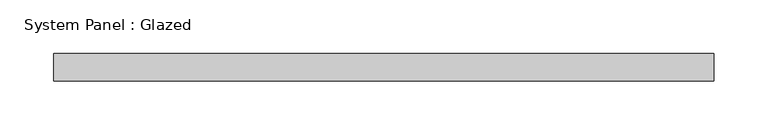
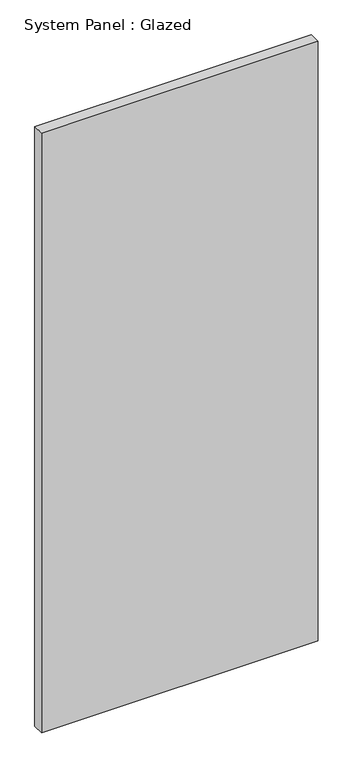
"""IFC4 building model written with IfcOpenShell, lengths in millimetres: plate geometry, System Panel : Glazed."""

from ifc_helpers import new_model, si_unit, origin, origin_with_axes, place, context, project, spatial, polyline, outline, extrude, source, transform, mapped, element, save


def system_panel_glazed_4048e9f5(model_context):
    return source(origin(), model_context, "Body", "SweptSolid", [
        extrude(outline(polyline([(306.3875, 19.05), (-306.3875, 19.05), (-306.3875, 44.45), (306.3875, 44.45), (306.3875, 19.05)])), origin_with_axes(), (0.0, 0.0, 1.0), 1404.3368617),
    ])


if __name__ == "__main__":
    model = new_model("IFC4")
    model_context = context("Model", 3, world=origin())
    ifc_project = project(units=[si_unit("LENGTHUNIT", "METRE", prefix="MILLI")], contexts=[model_context])
    site = spatial("IfcSite", under=ifc_project)
    building = spatial("IfcBuilding", under=site)
    placement = place(None, origin())
    system_panel_glazed_shape = system_panel_glazed_4048e9f5(model_context)
    element("IfcPlate", 1, ObjectType="System Panel : Glazed", at=placement, inside=building, context=model_context, shape_type="MappedRepresentation", body=[
        mapped(system_panel_glazed_shape, transform((0.0, 0.0, 0.0), x_axis=(1.0, 0.0, 0.0), y_axis=(0.0, 1.0, 0.0), z_axis=(0.0, 0.0, 1.0))),
    ])
    save(model, "model.ifc")

# Revit data of these elements
# Type "System Panel : Glazed"
#   Construction Type Id = "GSP4R"
#   Analytic Construction = "1/8 in Pilkington single glazing"
#   Visual Light Transmittance = 0.9
#   Solar Heat Gain Coefficient = 0.86
#   Heat Transfer Coefficient (U) = 1.18115 BTU/(h·ft²·°F)
#   Define Thermal Properties by = 1
# Element 1 (IfcPlate, "System Panel : Glazed")
#   Materials on its faces: "Glass"
# Materials
#   "Glass": class "Glass", colour RGB 0 128 192, transparency 0.75, Description = "Soda Lime Glass", Cost = 0
